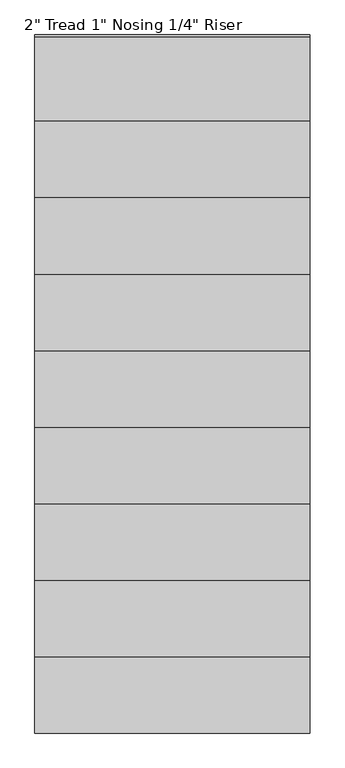
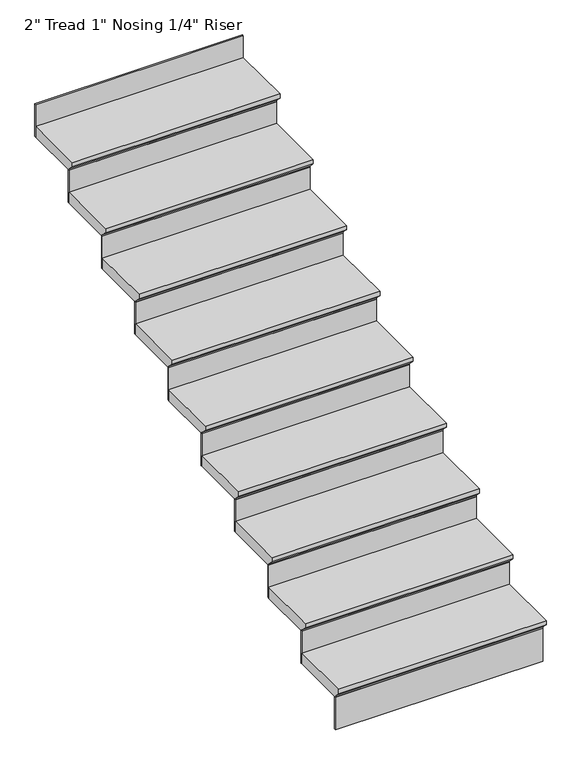
"""IFC4 building model written with IfcOpenShell, lengths in millimetres: stair flight geometry."""

from ifc_helpers import new_model, si_unit, frame, origin, place, context, project, spatial, polyline, outline, extrude, source, transform, mapped, element, save


def stair_flight_6110c9a1(model_context):
    return source(origin(), model_context, "Body", "SweptSolid", [
        extrude(outline(polyline([(-6527.0593836, 4876.8), (-6247.6593836, 4876.8), (-6247.6593836, 4826.0), (-6501.6593836, 4826.0), (-6501.6593836, 4832.35), (-6527.0593836, 4857.75), (-6527.0593836, 4876.8)])), frame((-5280.3137331, 0.0, 0.0), z_axis=(1.0, 0.0, 0.0), x_axis=(0.0, 1.0, 0.0)), (0.0, 0.0, 1.0), 914.4),
        extrude(outline(polyline([(-4365.9137331, -6495.3093836), (-4365.9137331, -6501.6593836), (-5280.3137331, -6501.6593836), (-5280.3137331, -6495.3093836), (-4365.9137331, -6495.3093836)])), frame((0.0, 0.0, 4673.6), z_axis=(0.0, 0.0, 1.0), x_axis=(1.0, 0.0, 0.0)), (0.0, 0.0, 1.0), 152.4),
        extrude(outline(polyline([(-4365.9137331, -6241.3093836), (-4365.9137331, -6247.6593836), (-5280.3137331, -6247.6593836), (-5280.3137331, -6241.3093836), (-4365.9137331, -6241.3093836)])), frame((0.0, 0.0, 4826.0), z_axis=(0.0, 0.0, 1.0), x_axis=(1.0, 0.0, 0.0)), (0.0, 0.0, 1.0), 152.4),
        extrude(outline(polyline([(-6273.0593836, 5029.2), (-5993.6593836, 5029.2), (-5993.6593836, 4978.4), (-6247.6593836, 4978.4), (-6247.6593836, 4984.75), (-6273.0593836, 5010.15), (-6273.0593836, 5029.2)])), frame((-5280.3137331, 0.0, 0.0), z_axis=(1.0, 0.0, 0.0), x_axis=(0.0, 1.0, 0.0)), (0.0, 0.0, 1.0), 914.4),
        extrude(outline(polyline([(-4365.9137331, -5987.3093836), (-4365.9137331, -5993.6593836), (-5280.3137331, -5993.6593836), (-5280.3137331, -5987.3093836), (-4365.9137331, -5987.3093836)])), frame((0.0, 0.0, 4978.4), z_axis=(0.0, 0.0, 1.0), x_axis=(1.0, 0.0, 0.0)), (0.0, 0.0, 1.0), 152.4),
        extrude(outline(polyline([(-6019.0593836, 5181.6), (-5739.6593836, 5181.6), (-5739.6593836, 5130.8), (-5993.6593836, 5130.8), (-5993.6593836, 5137.15), (-6019.0593836, 5162.55), (-6019.0593836, 5181.6)])), frame((-5280.3137331, 0.0, 0.0), z_axis=(1.0, 0.0, 0.0), x_axis=(0.0, 1.0, 0.0)), (0.0, 0.0, 1.0), 914.4),
        extrude(outline(polyline([(-4365.9137331, -5733.3093836), (-4365.9137331, -5739.6593836), (-5280.3137331, -5739.6593836), (-5280.3137331, -5733.3093836), (-4365.9137331, -5733.3093836)])), frame((0.0, 0.0, 5130.8), z_axis=(0.0, 0.0, 1.0), x_axis=(1.0, 0.0, 0.0)), (0.0, 0.0, 1.0), 152.4),
        extrude(outline(polyline([(-5765.0593836, 5334.0), (-5485.6593836, 5334.0), (-5485.6593836, 5283.2), (-5739.6593836, 5283.2), (-5739.6593836, 5289.55), (-5765.0593836, 5314.95), (-5765.0593836, 5334.0)])), frame((-5280.3137331, 0.0, 0.0), z_axis=(1.0, 0.0, 0.0), x_axis=(0.0, 1.0, 0.0)), (0.0, 0.0, 1.0), 914.4),
        extrude(outline(polyline([(-4365.9137331, -5479.3093836), (-4365.9137331, -5485.6593836), (-5280.3137331, -5485.6593836), (-5280.3137331, -5479.3093836), (-4365.9137331, -5479.3093836)])), frame((0.0, 0.0, 5283.2), z_axis=(0.0, 0.0, 1.0), x_axis=(1.0, 0.0, 0.0)), (0.0, 0.0, 1.0), 152.4),
        extrude(outline(polyline([(-5511.0593836, 5486.4), (-5231.6593836, 5486.4), (-5231.6593836, 5435.6), (-5485.6593836, 5435.6), (-5485.6593836, 5441.95), (-5511.0593836, 5467.35), (-5511.0593836, 5486.4)])), frame((-5280.3137331, 0.0, 0.0), z_axis=(1.0, 0.0, 0.0), x_axis=(0.0, 1.0, 0.0)), (0.0, 0.0, 1.0), 914.4),
        extrude(outline(polyline([(-4365.9137331, -5225.3093836), (-4365.9137331, -5231.6593836), (-5280.3137331, -5231.6593836), (-5280.3137331, -5225.3093836), (-4365.9137331, -5225.3093836)])), frame((0.0, 0.0, 5435.6), z_axis=(0.0, 0.0, 1.0), x_axis=(1.0, 0.0, 0.0)), (0.0, 0.0, 1.0), 152.4),
        extrude(outline(polyline([(-5257.0593836, 5638.8), (-4977.6593836, 5638.8), (-4977.6593836, 5588.0), (-5231.6593836, 5588.0), (-5231.6593836, 5594.35), (-5257.0593836, 5619.75), (-5257.0593836, 5638.8)])), frame((-5280.3137331, 0.0, 0.0), z_axis=(1.0, 0.0, 0.0), x_axis=(0.0, 1.0, 0.0)), (0.0, 0.0, 1.0), 914.4),
        extrude(outline(polyline([(-4365.9137331, -4971.3093836), (-4365.9137331, -4977.6593836), (-5280.3137331, -4977.6593836), (-5280.3137331, -4971.3093836), (-4365.9137331, -4971.3093836)])), frame((0.0, 0.0, 5588.0), z_axis=(0.0, 0.0, 1.0), x_axis=(1.0, 0.0, 0.0)), (0.0, 0.0, 1.0), 152.4),
        extrude(outline(polyline([(-5003.0593836, 5791.2), (-4723.6593836, 5791.2), (-4723.6593836, 5740.4), (-4977.6593836, 5740.4), (-4977.6593836, 5746.75), (-5003.0593836, 5772.15), (-5003.0593836, 5791.2)])), frame((-5280.3137331, 0.0, 0.0), z_axis=(1.0, 0.0, 0.0), x_axis=(0.0, 1.0, 0.0)), (0.0, 0.0, 1.0), 914.4),
        extrude(outline(polyline([(-4365.9137331, -4717.3093836), (-4365.9137331, -4723.6593836), (-5280.3137331, -4723.6593836), (-5280.3137331, -4717.3093836), (-4365.9137331, -4717.3093836)])), frame((0.0, 0.0, 5740.4), z_axis=(0.0, 0.0, 1.0), x_axis=(1.0, 0.0, 0.0)), (0.0, 0.0, 1.0), 152.4),
        extrude(outline(polyline([(-4749.0593836, 5943.6), (-4469.6593836, 5943.6), (-4469.6593836, 5892.8), (-4723.6593836, 5892.8), (-4723.6593836, 5899.15), (-4749.0593836, 5924.55), (-4749.0593836, 5943.6)])), frame((-5280.3137331, 0.0, 0.0), z_axis=(1.0, 0.0, 0.0), x_axis=(0.0, 1.0, 0.0)), (0.0, 0.0, 1.0), 914.4),
        extrude(outline(polyline([(-4365.9137331, -4463.3093836), (-4365.9137331, -4469.6593836), (-5280.3137331, -4469.6593836), (-5280.3137331, -4463.3093836), (-4365.9137331, -4463.3093836)])), frame((0.0, 0.0, 5892.8), z_axis=(0.0, 0.0, 1.0), x_axis=(1.0, 0.0, 0.0)), (0.0, 0.0, 1.0), 152.4),
        extrude(outline(polyline([(-4365.9137331, -4209.3093836), (-4365.9137331, -4215.6593836), (-5280.3137331, -4215.6593836), (-5280.3137331, -4209.3093836), (-4365.9137331, -4209.3093836)])), frame((0.0, 0.0, 6045.2), z_axis=(0.0, 0.0, 1.0), x_axis=(1.0, 0.0, 0.0)), (0.0, 0.0, 1.0), 152.4),
        extrude(outline(polyline([(-4495.0593836, 6096.0), (-4215.6593836, 6096.0), (-4215.6593836, 6045.2), (-4469.6593836, 6045.2), (-4469.6593836, 6051.55), (-4495.0593836, 6076.95), (-4495.0593836, 6096.0)])), frame((-5280.3137331, 0.0, 0.0), z_axis=(1.0, 0.0, 0.0), x_axis=(0.0, 1.0, 0.0)), (0.0, 0.0, 1.0), 914.4),
    ])


if __name__ == "__main__":
    model = new_model("IFC4")
    model_context = context("Model", 3, world=origin())
    ifc_project = project(units=[si_unit("LENGTHUNIT", "METRE", prefix="MILLI")], contexts=[model_context])
    site = spatial("IfcSite", under=ifc_project)
    building = spatial("IfcBuilding", under=site)
    placement = place(None, origin())
    stair_flight_shape = stair_flight_6110c9a1(model_context)
    element("IfcStairFlight", 1, ObjectType="2\" Tread 1\" Nosing 1/4\" Riser", at=placement, inside=building, context=model_context, shape_type="MappedRepresentation", body=[
        mapped(stair_flight_shape, transform((0.0, 0.0, 0.0), x_axis=(1.0, 0.0, 0.0), y_axis=(0.0, 1.0, 0.0), z_axis=(0.0, 0.0, 1.0))),
    ])
    save(model, "model.ifc")
